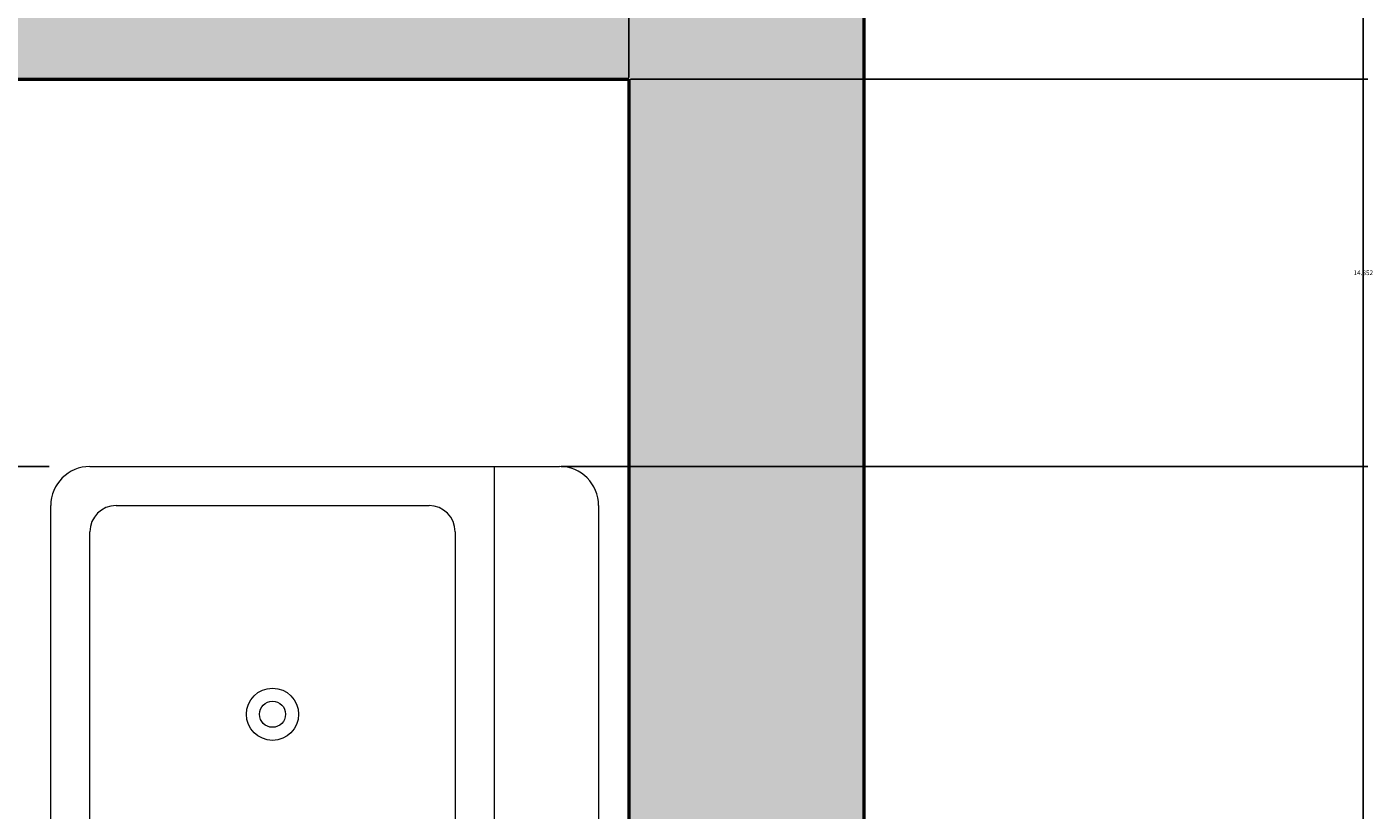
# Model space of a CAD drawing. Units: inches. Extents: x 2307 to 2544, y 2171 to 2540.
# Tile 39 of 52: x 2493 to 2544, y 2407 to 2438. Entities that reach past the tile are written whole.
import ezdxf

# ---------------------------------------------------------------- set-up
doc = ezdxf.new("R2010")
doc.units = ezdxf.units.IN
for name, color, linetype, lineweight in [('A-ANNO-DIMS', 2, 'Continuous', 18), ('A-FLOR-FIXT', 9, 'Continuous', 18), ('A-WALL', 7, 'Continuous', 50)]:
    doc.layers.add(name, color=color, linetype=linetype, lineweight=lineweight)
doc.layers.add('A-WALL-PATT', color=18, linetype='Continuous', lineweight=13, true_color=0x000000)
doc.styles.get("Standard").update_dxf_attribs({"font": 'arial.ttf'})
doc.dimstyles.get("Standard").update_dxf_attribs({"dimtxt": 0.18, "dimasz": 0.18, "dimexe": 0.18, "dimexo": 0.0625, "dimgap": 0.09, "dimtad": 0, "dimtih": 1, "dimtoh": 1, "dimdec": 4, "dimzin": 0, "dimdsep": 46, "dimtxsty": 'Standard', "dimcen": 0.09, "dimadec": 0, "dimazin": 0, "dimtfac": 1, "dimtdec": 4, "dimtofl": 0, "dimtmove": 0, "dimatfit": 3, "dimfxl": 1, "dimtolj": 1, "dimtzin": 0, "dimarcsym": 0})

# ---------------------------------------------------------------- blocks, each defined once
blk = doc.blocks.new('Sink-double - 36 in top')
blk.add_line((-18, -4), (18, -4))
for points in [[(-16.5, 0), (16.5, 0)], [(-18, -19.5), (-18, -1.5)], [(-15.5, -5.5), (-1.75, -5.5)], [(-16.5, -18.5), (-16.5, -6.5)], [(-1.75, -19.5), (-15.5, -19.5)], [(16.5, -21), (-16.5, -21)]]:
    blk.add_lwpolyline(points)
for radius in [1, 0.5]:
    blk.add_circle((-8.5, -12.5), radius)
for centre, radius, start, end in [((-16.5, -1.5), 1.5, 90, 180), ((-15.5, -6.5), 1, 90, 180), ((-15.5, -18.5), 1, 180, 270), ((-16.5, -19.5), 1.5, 180, 270)]:
    blk.add_arc(centre, radius, start, end)
blk = doc.blocks.new('*D32')
at = {"layer": 'A-ANNO-DIMS', "color": 0, "lineweight": -2, "transparency": 16777216}
for p, q in [((2493.473, 2420.657), (2487.956, 2420.657)), ((2488.136, 2420.477), (2488.136, 2402.84)), ((2488.136, 2384.837), (2488.136, 2402.474)), ((2493.473, 2384.657), (2487.956, 2384.657))]:
    blk.add_line(p, q, dxfattribs=at)
at = {"layer": 'A-ANNO-DIMS', "color": 0, "transparency": 16777216}
for points in [[(2488.106, 2420.477), (2488.166, 2420.477), (2488.136, 2420.657)], [(2488.106, 2384.837), (2488.166, 2384.837), (2488.136, 2384.657)]]:
    blk.add_solid(points, dxfattribs=at)
at = {"layer": 'Defpoints', "color": 0, "transparency": 16777216}
for p in [(2493.536, 2420.657), (2488.136, 2384.657), (2493.536, 2384.657)]:
    blk.add_point(p, dxfattribs=at)
at = {"layer": 'A-ANNO-DIMS', "color": 0, "transparency": 16777216, "insert": (2488.136, 2402.657), "char_height": 0.18, "attachment_point": 5}
blk.add_mtext('\\A1;DOUBLE SINK 36', dxfattribs=at)
blk = doc.blocks.new('*D37')
at = {"layer": 'A-ANNO-DIMS', "color": 0, "lineweight": -2, "transparency": 16777216}
for p, q in [((2524.758, 2520.51), (2544.026, 2520.51)), ((2543.846, 2520.33), (2543.846, 2355.692)), ((2543.846, 2190.69), (2543.846, 2355.328)), ((2524.758, 2190.51), (2544.026, 2190.51))]:
    blk.add_line(p, q, dxfattribs=at)
at = {"layer": 'A-ANNO-DIMS', "color": 0, "transparency": 16777216}
for points in [[(2543.816, 2520.33), (2543.876, 2520.33), (2543.846, 2520.51)], [(2543.816, 2190.69), (2543.876, 2190.69), (2543.846, 2190.51)]]:
    blk.add_solid(points, dxfattribs=at)
at = {"layer": 'Defpoints', "color": 0, "transparency": 16777216}
for p in [(2524.696, 2520.51), (2543.846, 2520.51), (2524.696, 2190.51)]:
    blk.add_point(p, dxfattribs=at)
at = {"layer": 'A-ANNO-DIMS', "color": 0, "transparency": 16777216, "insert": (2543.846, 2355.51), "char_height": 0.18, "attachment_point": 5}
blk.add_mtext('\\A1;330', dxfattribs=at)
blk = doc.blocks.new('*D61')
at = {"layer": 'A-ANNO-DIMS', "color": 0, "lineweight": -2, "transparency": 16777216}
for p, q in [((2491.696, 2435.572), (2491.696, 2540.345)), ((2515.696, 2435.572), (2515.696, 2540.345)), ((2491.876, 2540.165), (2503.476, 2540.165)), ((2515.516, 2540.165), (2503.916, 2540.165))]:
    blk.add_line(p, q, dxfattribs=at)
at = {"layer": 'A-ANNO-DIMS', "color": 0, "transparency": 16777216}
for points in [[(2491.876, 2540.195), (2491.876, 2540.135), (2491.696, 2540.165)], [(2515.516, 2540.195), (2515.516, 2540.135), (2515.696, 2540.165)]]:
    blk.add_solid(points, dxfattribs=at)
at = {"layer": 'Defpoints', "color": 0, "transparency": 16777216}
for p in [(2515.696, 2540.165), (2491.696, 2435.51), (2515.696, 2435.51)]:
    blk.add_point(p, dxfattribs=at)
at = {"layer": 'A-ANNO-DIMS', "color": 0, "transparency": 16777216, "insert": (2503.696, 2540.165), "char_height": 0.18, "attachment_point": 5}
blk.add_mtext('\\A1;24', dxfattribs=at)
blk = doc.blocks.new('*D62')
at = {"layer": 'A-ANNO-DIMS', "color": 0, "lineweight": -2, "transparency": 16777216}
for p, q in [((2515.758, 2435.51), (2544.026, 2435.51)), ((2543.846, 2435.33), (2543.846, 2428.265)), ((2543.846, 2420.837), (2543.846, 2427.902)), ((2513.098, 2420.657), (2544.026, 2420.657))]:
    blk.add_line(p, q, dxfattribs=at)
at = {"layer": 'A-ANNO-DIMS', "color": 0, "transparency": 16777216}
for points in [[(2543.816, 2435.33), (2543.876, 2435.33), (2543.846, 2435.51)], [(2543.816, 2420.837), (2543.876, 2420.837), (2543.846, 2420.657)]]:
    blk.add_solid(points, dxfattribs=at)
at = {"layer": 'Defpoints', "color": 0, "transparency": 16777216}
for p in [(2515.696, 2435.51), (2513.036, 2420.657), (2543.846, 2420.657)]:
    blk.add_point(p, dxfattribs=at)
at = {"layer": 'A-ANNO-DIMS', "color": 0, "transparency": 16777216, "insert": (2543.846, 2428.083), "char_height": 0.18, "attachment_point": 5}
blk.add_mtext('\\A1;14.852', dxfattribs=at)

msp = doc.modelspace()

# ---------------------------------------------------------------- hatches: boundary and pattern name
at = {"layer": 'A-WALL-PATT'}
h = msp.add_hatch(color=256, dxfattribs=at)
h.dxf.hatch_style = 1
h.paths.add_polyline_path([(2433.6935, 2199.5096), (2415.6423, 2199.5096), (2415.6423, 2190.5096), (2433.7832, 2190.5096)], flags=17)
h.paths.add_polyline_path([(2367.6423, 2199.5096), (2335.6958, 2199.5096), (2335.6958, 2307.3983), (2326.6958, 2307.3983), (2326.6958, 2190.5096), (2367.6423, 2190.5096)])
h.paths.add_polyline_path([(2524.6958, 2520.5096), (2496.7832, 2520.5096), (2496.7832, 2515.5149), (2472.7832, 2515.5149), (2472.7832, 2520.5096), (2415.4028, 2520.5096), (2415.4028, 2511.5096), (2451.6958, 2511.5096), (2451.6958, 2439.5096), (2451.6958, 2391.5096), (2445.6958, 2391.5096), (2445.6958, 2387.5096), (2455.6958, 2387.5096), (2455.6958, 2435.5096), (2461.6958, 2435.5096), (2461.6958, 2439.5096), (2455.6958, 2439.5096), (2455.6958, 2511.5096), (2515.6958, 2511.5096), (2515.6958, 2439.5096), (2491.6958, 2439.5096), (2491.6958, 2435.5096), (2515.6958, 2435.5096), (2515.6958, 2319.5096), (2451.6958, 2319.5096), (2451.6958, 2281.5096), (2481.6958, 2281.5096), (2481.6958, 2225.5096), (2485.6958, 2225.5096), (2485.6958, 2285.5096), (2455.6958, 2285.5096), (2455.6958, 2315.5096), (2515.6958, 2315.5096), (2515.6958, 2199.5096), (2469.6952, 2199.5096), (2469.785, 2190.5096), (2524.6958, 2190.5096)])

# ---------------------------------------------------------------- linework, layer by layer
at = {"layer": 'A-WALL'}
for p, q in [((2491.6958, 2435.5096), (2515.6958, 2435.5096)), ((2515.6958, 2435.5096), (2515.6958, 2319.5096))]:
    msp.add_line(p, q, dxfattribs=at)
msp.add_lwpolyline([(2433.7832, 2190.5096), (2326.6958, 2190.5096), (2326.6958, 2520.5096), (2524.6958, 2520.5096), (2524.6958, 2190.5096), (2469.785, 2190.5096)], dxfattribs=at)

# ---------------------------------------------------------------- block references
at = {"layer": 'A-FLOR-FIXT', "rotation": 270}
msp.add_blockref('Sink-double - 36 in top', (2514.5356, 2402.6573), dxfattribs=at)

# ---------------------------------------------------------------- dimensions: what is measured, and where the dimension line sits
at = {"layer": 'A-ANNO-DIMS'}
dim = msp.add_linear_dim(base=(2515.6958, 2540.1649), p1=(2491.6958, 2435.5096), p2=(2515.6958, 2435.5096), dimstyle='Standard', override={"dimdec": 0, "dimlfac": 1, "dimrnd": 0, "dimzin": 0, "dimdsep": 46, "dimlunit": 2}, dxfattribs=at)
dim.commit()
dim.dimension.update_dxf_attribs({"geometry": '*D61', "text_midpoint": (2503.6958, 2540.1649)})
for base, p1, p2, override, picture, middle in [((2543.8458, 2520.5096), (2524.6958, 2190.5096), (2524.6958, 2520.5096), {"dimdec": 0, "dimlfac": 1, "dimrnd": 0, "dimzin": 0, "dimdsep": 46, "dimlunit": 2}, '*D37', (2543.8458, 2355.5096)), ((2543.8458, 2420.6573), (2515.6958, 2435.5096), (2513.0356, 2420.6573), {"dimdec": 3, "dimlfac": 1, "dimrnd": 0, "dimzin": 0, "dimdsep": 46, "dimlunit": 2}, '*D62', (2543.8458, 2428.0834))]:
    dim = msp.add_linear_dim(base=base, p1=p1, p2=p2, angle=90, dimstyle='Standard', override=override, dxfattribs=at)
    dim.commit()
    dim.dimension.update_dxf_attribs({"geometry": picture, "text_midpoint": middle})
dim = msp.add_linear_dim(base=(2488.1356, 2384.6573), p1=(2493.5356, 2420.6573), p2=(2493.5356, 2384.6573), angle=270, text='DOUBLE SINK <>', dimstyle='Standard', override={"dimdec": 0, "dimlfac": 1, "dimrnd": 0, "dimzin": 0, "dimdsep": 46, "dimlunit": 2}, dxfattribs=at)
dim.commit()
dim.dimension.update_dxf_attribs({"geometry": '*D32', "text_midpoint": (2488.1356, 2402.6573)})

doc.saveas('drawing.dxf')
